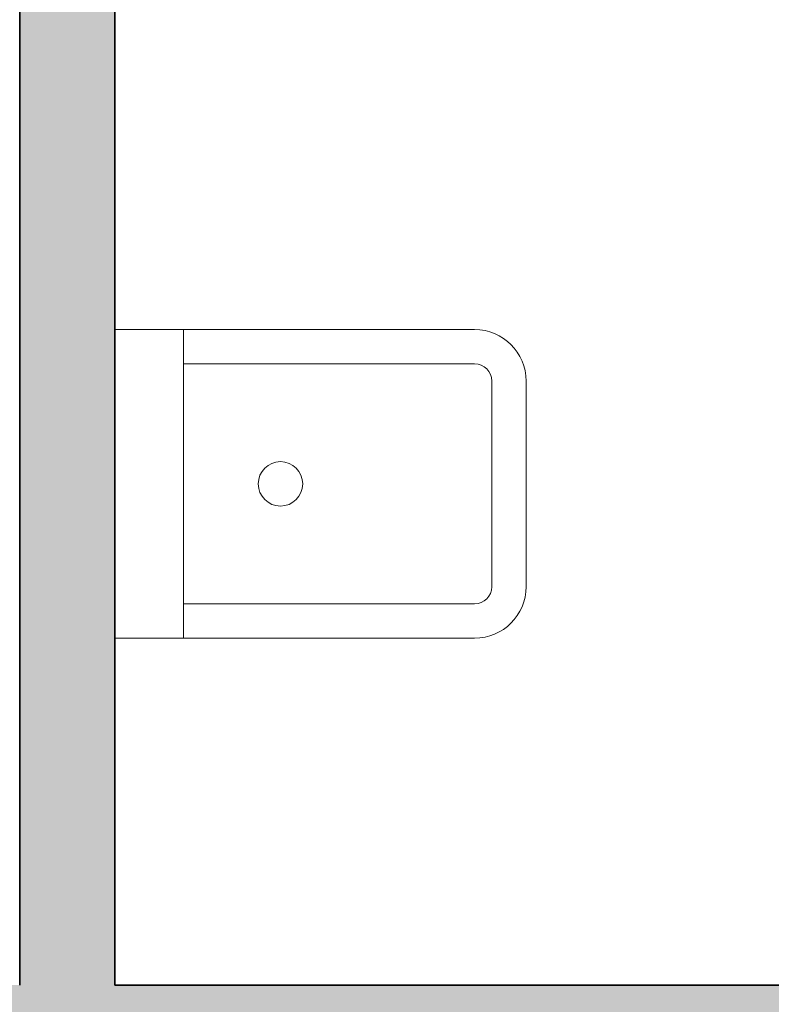
# Model space of a CAD drawing. Units: inches. Extents: x 2696 to 3240, y 1564 to 2310.
# Tile 28 of 76: x 3102 to 3138, y 1699 to 1745. Entities that reach past the tile are written whole.
import ezdxf

# ---------------------------------------------------------------- set-up
doc = ezdxf.new("R2010")
doc.units = ezdxf.units.IN
for name, color, linetype, lineweight in [('A-ANNO-DIMS', 3, 'Continuous', 18), ('A-FLOR-FIXT', 8, 'Continuous', 18), ('A-FURN', 251, 'Continuous', 13), ('A-WALL', 7, 'Continuous', 35), ('A-WALL-PATT', 9, 'Continuous', 13)]:
    doc.layers.add(name, color=color, linetype=linetype, lineweight=lineweight)
doc.styles.add('TIMES NEW', font='times.ttf')
doc.dimstyles.new('Siddhuu', dxfattribs={"dimtxt": 6, "dimasz": 2.5, "dimexe": 1.25, "dimexo": 0.625, "dimtad": 1, "dimdec": 1, "dimlunit": 4, "dimtxsty": 'TIMES NEW', "dimcen": 2.5, "dimclrd": 256, "dimclre": 1, "dimclrt": 7, "dimadec": 0, "dimazin": 0, "dimtfac": 1, "dimtdec": 1, "dimtmove": 0, "dimatfit": 3, "dimfxl": 1, "dimtolj": 1, "dimlwd": -1, "dimarcsym": 0})

# ---------------------------------------------------------------- blocks, each defined once
blk = doc.blocks.new('WC')
at = {"layer": 'A-FURN'}
for p, q in [((0, 14.59), (-17.022, 14.59)), ((-3.242, 14.59), (-3.242, 0)), ((-3.242, 12.969), (-17.022, 12.969)), ((-19.454, 2.432), (-19.454, 12.159)), ((-17.833, 2.432), (-17.833, 12.159)), ((-3.242, 1.621), (-17.022, 1.621)), ((0, 0), (-17.022, 0))]:
    blk.add_line(p, q, dxfattribs=at)
blk.add_circle((-7.836, 7.295), 1.051, dxfattribs=at)
for centre, radius, start, end in [((-17.022, 12.159), 2.432, 90, 180), ((-17.022, 12.159), 0.811, 90, 180), ((-17.022, 2.432), 2.432, 180, 270), ((-17.022, 2.432), 0.811, 180, 270)]:
    blk.add_arc(centre, radius, start, end, dxfattribs=at)
blk = doc.blocks.new('*D51')
at = {"layer": 'A-ANNO-DIMS', "color": 1, "lineweight": -2, "transparency": 16777216}
for p, q in [((3016.611, 1979.576), (3016.611, 1568.951)), ((3148.611, 1979.576), (3148.611, 1568.951))]:
    blk.add_line(p, q, dxfattribs=at)
at = {"layer": 'A-ANNO-DIMS', "transparency": 16777216}
blk.add_line((3019.111, 1570.201), (3146.111, 1570.201), dxfattribs=at)
for points in [[(3019.111, 1570.618), (3019.111, 1569.784), (3016.611, 1570.201)], [(3146.111, 1570.618), (3146.111, 1569.784), (3148.611, 1570.201)]]:
    blk.add_solid(points, dxfattribs=at)
at = {"layer": 'Defpoints', "color": 0, "transparency": 16777216}
for p in [(3016.611, 1980.201), (3148.611, 1980.201), (3148.611, 1570.201)]:
    blk.add_point(p, dxfattribs=at)
at = {"layer": 'A-ANNO-DIMS', "color": 7, "transparency": 16777216, "insert": (3082.611, 1573.878), "char_height": 6, "attachment_point": 5, "style": 'TIMES NEW'}
blk.add_mtext('\\A1;11\'-0"', dxfattribs=at)
blk = doc.blocks.new('*D56')
at = {"layer": 'A-ANNO-DIMS', "color": 1, "lineweight": -2, "transparency": 16777216}
for p, q in [((2966.334, 1884.201), (3235.861, 1884.201)), ((2966.334, 1665.201), (3235.861, 1665.201))]:
    blk.add_line(p, q, dxfattribs=at)
at = {"layer": 'A-ANNO-DIMS', "transparency": 16777216}
blk.add_line((3234.611, 1667.701), (3234.611, 1881.701), dxfattribs=at)
for points in [[(3234.195, 1881.701), (3235.028, 1881.701), (3234.611, 1884.201)], [(3234.195, 1667.701), (3235.028, 1667.701), (3234.611, 1665.201)]]:
    blk.add_solid(points, dxfattribs=at)
at = {"layer": 'Defpoints', "color": 0, "transparency": 16777216}
for p in [(2965.709, 1884.201), (3234.611, 1884.201), (2965.709, 1665.201)]:
    blk.add_point(p, dxfattribs=at)
at = {"layer": 'A-ANNO-DIMS', "color": 7, "transparency": 16777216, "insert": (3230.934, 1774.701), "char_height": 6, "attachment_point": 5, "rotation": 90, "style": 'TIMES NEW'}
blk.add_mtext('\\A1;18\'-3"', dxfattribs=at)

msp = doc.modelspace()

# ---------------------------------------------------------------- hatches: boundary and pattern name
at = {"layer": 'A-WALL-PATT', "transparency": 33554556}
h = msp.add_hatch(color=256, dxfattribs=at)
h.dxf.hatch_style = 1
h.paths.add_polyline_path([(2879.111, 2253.201), (2905.91, 2253.201), (2905.91, 2262.201), (2841.889, 2262.201), (2841.889, 2253.201), (2870.111, 2253.201), (2870.111, 2176.601), (2965.709, 2176.601), (2965.709, 2206.701), (2973.583, 2206.701), (2973.583, 2215.701), (2965.709, 2215.701), (2965.709, 2262.201), (2929.91, 2262.201), (2929.91, 2253.201), (2956.709, 2253.201), (2956.709, 2185.601), (2879.111, 2185.601)])
h.paths.add_polyline_path([(2782.834, 2262.201), (2745.611, 2262.201), (2745.611, 2228.729), (2754.611, 2228.729), (2754.611, 2253.201), (2782.834, 2253.201)])
h.paths.add_polyline_path([(2754.611, 2136.201), (2965.709, 2136.201), (2965.709, 2145.201), (2879.111, 2145.201), (2879.111, 2147.074), (2877.34, 2147.074), (2870.111, 2147.074), (2870.111, 2145.201), (2754.611, 2145.201), (2754.611, 2169.674), (2745.611, 2169.674), (2745.611, 2000.201), (2754.611, 2000.201), (2754.611, 2019.201), (2849.083, 2019.201), (2849.083, 2023.701), (2841.209, 2023.701), (2841.209, 2051.827), (2836.709, 2051.827), (2836.709, 2023.701), (2754.611, 2023.701), (2754.611, 2091.201), (2836.709, 2091.201), (2836.709, 2087.827), (2841.209, 2087.827), (2841.209, 2095.701), (2754.611, 2095.701)])
h.paths.add_polyline_path([(2965.709, 2136.201), (2956.709, 2136.201), (2956.709, 2023.701), (2885.083, 2023.701), (2885.083, 2019.201), (2956.709, 2019.201), (2956.709, 1950.575), (2965.709, 1950.575), (2965.709, 1980.201), (2973.583, 1980.201), (2973.583, 1989.201), (2965.709, 1989.201)])
h.paths.add_polyline_path([(2754.611, 1906.701), (2880.209, 1906.701), (2884.709, 1906.701), (2956.709, 1906.701), (2956.709, 1792.701), (2944.709, 1792.701), (2944.709, 1783.701), (2956.709, 1783.701), (2956.709, 1740.201), (2884.709, 1740.201), (2884.709, 1783.701), (2896.709, 1783.701), (2896.709, 1792.701), (2884.709, 1792.701), (2884.709, 1846.701), (2880.209, 1846.701), (2880.209, 1740.201), (2754.611, 1740.201), (2754.611, 1777.201), (2745.611, 1777.201), (2745.611, 1692.701), (2754.611, 1692.701), (2754.611, 1731.201), (2956.709, 1731.201), (2956.709, 1723.327), (2965.709, 1723.327), (2965.709, 1884.201), (2973.583, 1884.201), (2973.583, 1893.201), (2965.709, 1893.201), (2965.709, 1914.575), (2956.709, 1914.575), (2956.709, 1911.201), (2754.611, 1911.201), (2754.611, 1930.201), (2745.611, 1930.201), (2745.611, 1817.201), (2754.611, 1817.201), (2754.611, 1854.201), (2826.611, 1854.201), (2826.611, 1868.827), (2822.111, 1868.827), (2822.111, 1858.701), (2754.611, 1858.701)])
h.paths.add_polyline_path([(2965.709, 1656.201), (3008.237, 1656.201), (3008.237, 1665.201), (2965.709, 1665.201), (2965.709, 1693.327), (2956.709, 1693.327), (2956.709, 1686.201), (2934.583, 1686.201), (2934.583, 1681.701), (2956.709, 1681.701), (2956.709, 1614.201), (2896.709, 1614.201), (2896.709, 1681.701), (2904.583, 1681.701), (2904.583, 1686.201), (2892.209, 1686.201), (2892.209, 1614.201), (2858.41, 1614.201), (2858.41, 1605.201), (2965.709, 1605.201)])
h.paths.add_polyline_path([(2788.41, 1614.201), (2754.611, 1614.201), (2754.611, 1652.701), (2745.611, 1652.701), (2745.611, 1605.201), (2788.41, 1605.201)])
h.paths.add_polyline_path([(3199.611, 1633.048), (3190.611, 1633.048), (3190.611, 1614.201), (3082.611, 1614.201), (3082.611, 1665.201), (3070.237, 1665.201), (3070.237, 1656.201), (3078.111, 1656.201), (3078.111, 1605.201), (3199.611, 1605.201)])
h.paths.add_polyline_path([(3199.611, 1702.048), (3190.611, 1702.048), (3190.611, 1699.701), (3106.611, 1699.701), (3106.611, 1747.701), (3190.611, 1747.701), (3190.611, 1752.201), (3082.611, 1752.201), (3082.611, 1760.075), (3078.111, 1760.075), (3078.111, 1747.701), (3102.111, 1747.701), (3102.111, 1699.701), (3078.111, 1699.701), (3078.111, 1695.201), (3190.611, 1695.201), (3190.611, 1676.355), (3199.611, 1676.355)])
h.paths.add_polyline_path([(3199.611, 1783.201), (3190.611, 1783.201), (3190.611, 1745.355), (3199.611, 1745.355)])
h.paths.add_polyline_path([(3082.611, 1884.201), (3190.611, 1884.201), (3190.611, 1853.201), (3199.611, 1853.201), (3199.611, 1901.701), (3190.611, 1901.701), (3190.611, 1893.201), (3005.583, 1893.201), (3005.583, 1891.281), (3005.583, 1884.201), (3078.111, 1884.201), (3078.111, 1792.075), (3082.611, 1792.075)])
h.paths.add_polyline_path([(3199.611, 1994.701), (3190.611, 1994.701), (3190.611, 1989.201), (3073.709, 1989.201), (3073.709, 2034.201), (3069.209, 2034.201), (3069.209, 1989.201), (3005.583, 1989.201), (3005.583, 1980.201), (3190.611, 1980.201), (3190.611, 1971.701), (3199.611, 1971.701)])
h.paths.add_polyline_path([(3199.611, 2155.201), (3190.611, 2155.201), (3190.611, 2064.701), (3199.611, 2064.701)])
h.paths.add_polyline_path([(3190.611, 2074.701), (3106.611, 2074.701), (3106.611, 2122.701), (3190.611, 2122.701), (3190.611, 2127.201), (3082.709, 2127.201), (3082.709, 2135.075), (3073.709, 2135.075), (3073.709, 2122.701), (3102.111, 2122.701), (3102.111, 2074.701), (3069.209, 2074.701), (3069.209, 2070.201), (3190.611, 2070.201)])
h.paths.add_polyline_path([(3082.709, 2253.201), (3190.611, 2253.201), (3190.611, 2225.201), (3199.611, 2225.201), (3199.611, 2262.201), (3073.709, 2262.201), (3073.709, 2215.701), (3035.583, 2215.701), (3035.583, 2206.701), (3073.709, 2206.701), (3073.709, 2171.075), (3082.709, 2171.075)])

# ---------------------------------------------------------------- linework, layer by layer
at = {"layer": 'A-WALL'}
for p, q in [((3102.111, 1699.701), (3102.111, 1747.701)), ((3106.611, 1699.701), (3106.611, 1747.701)), ((3106.611, 1699.701), (3190.611, 1699.701))]:
    msp.add_line(p, q, dxfattribs=at)

# ---------------------------------------------------------------- block references
at = {"layer": 'A-FLOR-FIXT', "xscale": -1}
msp.add_blockref('WC', (3106.611, 1716.108), dxfattribs=at)

# ---------------------------------------------------------------- dimensions: what is measured, and where the dimension line sits
at = {"layer": 'A-ANNO-DIMS'}
dim = msp.add_linear_dim(base=(3148.611, 1570.201), p1=(3016.611, 1980.201), p2=(3148.611, 1980.201), dimstyle='Siddhuu', override={"dimdec": 1, "dimlfac": 1, "dimrnd": 0, "dimzin": 1, "dimdsep": 46, "dimlunit": 4, "dimfrac": 2}, dxfattribs=at)
dim.commit()
dim.dimension.update_dxf_attribs({"geometry": '*D51', "text_midpoint": (3082.611, 1573.878)})
dim = msp.add_linear_dim(base=(3234.611, 1884.201), p1=(2965.709, 1665.201), p2=(2965.709, 1884.201), angle=90, dimstyle='Siddhuu', override={"dimdec": 1, "dimlfac": 1, "dimrnd": 0, "dimzin": 1, "dimdsep": 46, "dimlunit": 4, "dimfrac": 2}, dxfattribs=at)
dim.commit()
dim.dimension.update_dxf_attribs({"geometry": '*D56', "text_midpoint": (3230.934, 1774.701)})

doc.saveas('drawing.dxf')
